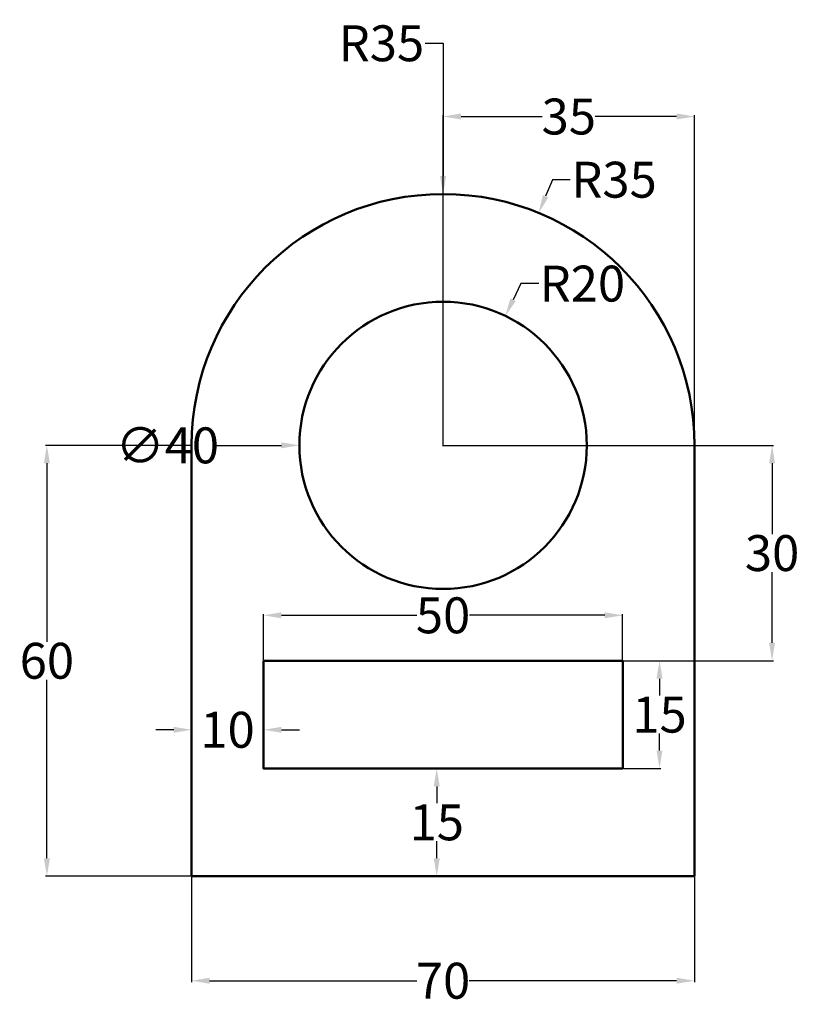
# Model space of a CAD drawing. Units: millimetres. Extents: x -34 to 74, y -57 to 80.
import ezdxf

# ---------------------------------------------------------------- set-up
doc = ezdxf.new("R2010")
doc.units = ezdxf.units.MM
doc.header["$MEASUREMENT"] = 0
doc.layers.add('M-DIMS', color=2, linetype='Continuous', lineweight=25)
doc.layers.add('M-OUTL', color=7, linetype='Continuous', lineweight=50)
doc.styles.get("Standard").update_dxf_attribs({"font": 'arial.ttf'})
doc.dimstyles.get("Standard").update_dxf_attribs({"dimtxt": 5, "dimasz": 2.5, "dimexe": 0.18, "dimexo": 0.1, "dimgap": 0.09, "dimtad": 0, "dimtih": 1, "dimtoh": 1, "dimdec": 4, "dimdsep": 46, "dimtxsty": 'Standard', "dimcen": 0.09, "dimclrd": 2, "dimclre": 2, "dimclrt": 2, "dimadec": 0, "dimazin": 0, "dimtfac": 1, "dimtdec": 4, "dimtofl": 0, "dimtmove": 0, "dimatfit": 3, "dimfxl": 1, "dimtfillclr": 2, "dimtolj": 1, "dimtzin": 0, "dimarcsym": 0})

# ---------------------------------------------------------------- blocks, each defined once
blk = doc.blocks.new('*D1')
at = {"layer": 'Defpoints', "color": 0, "transparency": 16777216}
for p in [(-10.41, -39.16), (59.59, -39.16), (59.59, -53.72)]:
    blk.add_point(p, dxfattribs=at)
at = {"layer": 'M-DIMS', "color": 0, "lineweight": -2, "transparency": 16777216}
for p, q in [((-10.41, -39.26), (-10.41, -53.9)), ((59.59, -39.26), (59.59, -53.9)), ((-7.91, -53.72), (20.95, -53.72)), ((57.09, -53.72), (28.23, -53.72))]:
    blk.add_line(p, q, dxfattribs=at)
at = {"layer": 'M-DIMS', "color": 0, "transparency": 16777216}
for points in [[(-7.91, -53.31), (-7.91, -54.14), (-10.41, -53.72)], [(57.09, -53.31), (57.09, -54.14), (59.59, -53.72)]]:
    blk.add_solid(points, dxfattribs=at)
at = {"layer": 'M-DIMS', "color": 0, "transparency": 16777216, "insert": (24.59, -53.72), "char_height": 5, "attachment_point": 5}
blk.add_mtext('\\A1;70', dxfattribs=at)
blk = doc.blocks.new('*D2')
at = {"layer": 'Defpoints', "color": 0, "transparency": 16777216}
for p in [(-30.56, 20.84), (-10.41, 20.84), (-10.41, -39.16)]:
    blk.add_point(p, dxfattribs=at)
at = {"layer": 'M-DIMS', "color": 0, "lineweight": -2, "transparency": 16777216}
for p, q in [((-10.51, 20.84), (-30.74, 20.84)), ((-30.56, 18.34), (-30.56, -6.51)), ((-30.56, -36.66), (-30.56, -11.8)), ((-10.51, -39.16), (-30.74, -39.16))]:
    blk.add_line(p, q, dxfattribs=at)
at = {"layer": 'M-DIMS', "color": 0, "transparency": 16777216}
for points in [[(-30.97, 18.34), (-30.14, 18.34), (-30.56, 20.84)], [(-30.97, -36.66), (-30.14, -36.66), (-30.56, -39.16)]]:
    blk.add_solid(points, dxfattribs=at)
at = {"layer": 'M-DIMS', "color": 0, "transparency": 16777216, "insert": (-30.56, -9.16), "char_height": 5, "attachment_point": 5}
blk.add_mtext('\\A1;60', dxfattribs=at)
blk = doc.blocks.new('*D3')
at = {"layer": 'Defpoints', "color": 0, "transparency": 16777216}
for p in [(49.59, -2.83), (-0.41, -9.16), (49.59, -9.16)]:
    blk.add_point(p, dxfattribs=at)
at = {"layer": 'M-DIMS', "color": 0, "lineweight": -2, "transparency": 16777216}
for p, q in [((-0.41, -9.06), (-0.41, -2.65)), ((49.59, -9.06), (49.59, -2.65)), ((2.09, -2.83), (20.93, -2.83)), ((47.09, -2.83), (28.25, -2.83))]:
    blk.add_line(p, q, dxfattribs=at)
at = {"layer": 'M-DIMS', "color": 0, "transparency": 16777216}
for points in [[(2.09, -2.41), (2.09, -3.24), (-0.41, -2.83)], [(47.09, -2.41), (47.09, -3.24), (49.59, -2.83)]]:
    blk.add_solid(points, dxfattribs=at)
at = {"layer": 'M-DIMS', "color": 0, "transparency": 16777216, "insert": (24.59, -2.83), "char_height": 5, "attachment_point": 5}
blk.add_mtext('\\A1;50', dxfattribs=at)
blk = doc.blocks.new('*D4')
at = {"layer": 'Defpoints', "color": 0, "transparency": 16777216}
for p in [(-10.41, -16.66), (-0.41, -16.66), (-10.41, -18.77)]:
    blk.add_point(p, dxfattribs=at)
at = {"layer": 'M-DIMS', "color": 0, "lineweight": -2, "transparency": 16777216}
for p, q in [((-10.41, -16.76), (-10.41, -18.95)), ((-0.41, -16.76), (-0.41, -18.95)), ((-12.91, -18.77), (-15.41, -18.77)), ((2.09, -18.77), (4.59, -18.77))]:
    blk.add_line(p, q, dxfattribs=at)
at = {"layer": 'M-DIMS', "color": 0, "transparency": 16777216}
for points in [[(-12.91, -18.36), (-12.91, -19.19), (-10.41, -18.77)], [(2.09, -18.36), (2.09, -19.19), (-0.41, -18.77)]]:
    blk.add_solid(points, dxfattribs=at)
at = {"layer": 'M-DIMS', "color": 0, "transparency": 16777216, "insert": (-5.41, -18.77), "char_height": 5, "attachment_point": 5}
blk.add_mtext('\\A1;10', dxfattribs=at)
blk = doc.blocks.new('*D5')
at = {"layer": 'Defpoints', "color": 0, "transparency": 16777216}
for p in [(24.59, -24.16), (23.71, -39.16), (24.59, -39.16)]:
    blk.add_point(p, dxfattribs=at)
at = {"layer": 'M-DIMS', "color": 0, "lineweight": -2, "transparency": 16777216}
for p, q in [((24.49, -24.16), (23.53, -24.16)), ((23.71, -26.66), (23.71, -29.01)), ((23.71, -36.66), (23.71, -34.3)), ((24.49, -39.16), (23.53, -39.16))]:
    blk.add_line(p, q, dxfattribs=at)
at = {"layer": 'M-DIMS', "color": 0, "transparency": 16777216}
for points in [[(23.29, -26.66), (24.13, -26.66), (23.71, -24.16)], [(23.29, -36.66), (24.13, -36.66), (23.71, -39.16)]]:
    blk.add_solid(points, dxfattribs=at)
at = {"layer": 'M-DIMS', "color": 0, "transparency": 16777216, "insert": (23.71, -31.66), "char_height": 5, "attachment_point": 5}
blk.add_mtext('\\A1;15', dxfattribs=at)
blk = doc.blocks.new('*D6')
at = {"layer": 'Defpoints', "color": 0, "transparency": 16777216}
for p in [(49.59, -9.16), (49.59, -24.16), (54.72, -24.16)]:
    blk.add_point(p, dxfattribs=at)
at = {"layer": 'M-DIMS', "color": 0, "lineweight": -2, "transparency": 16777216}
for p, q in [((49.69, -9.16), (54.9, -9.16)), ((54.72, -11.66), (54.72, -14.01)), ((54.72, -21.66), (54.72, -19.3)), ((49.69, -24.16), (54.9, -24.16))]:
    blk.add_line(p, q, dxfattribs=at)
at = {"layer": 'M-DIMS', "color": 0, "transparency": 16777216}
for points in [[(54.3, -11.66), (55.13, -11.66), (54.72, -9.16)], [(54.3, -21.66), (55.13, -21.66), (54.72, -24.16)]]:
    blk.add_solid(points, dxfattribs=at)
at = {"layer": 'M-DIMS', "color": 0, "transparency": 16777216, "insert": (54.72, -16.66), "char_height": 5, "attachment_point": 5}
blk.add_mtext('\\A1;15', dxfattribs=at)
blk = doc.blocks.new('*D7')
at = {"layer": 'Defpoints', "color": 0, "transparency": 16777216}
for p in [(33.26, 38.87), (24.59, 20.84)]:
    blk.add_point(p, dxfattribs=at)
at = {"layer": 'M-DIMS', "color": 0, "lineweight": -2, "transparency": 16777216}
for p, q in [((35.42, 43.37), (34.34, 41.12)), ((37.92, 43.37), (35.42, 43.37)), ((24.5, 20.84), (24.68, 20.84)), ((24.59, 20.75), (24.59, 20.93))]:
    blk.add_line(p, q, dxfattribs=at)
at = {"layer": 'M-DIMS', "color": 0, "transparency": 16777216}
blk.add_solid([(33.96, 41.3), (34.72, 40.94), (33.26, 38.87)], dxfattribs=at)
at = {"layer": 'M-DIMS', "color": 0, "transparency": 16777216, "insert": (43.98, 43.37), "char_height": 5, "attachment_point": 5}
blk.add_mtext('\\A1;R20', dxfattribs=at)
blk = doc.blocks.new('*D8')
at = {"layer": 'Defpoints', "color": 0, "transparency": 16777216}
for p in [(37.9, 53.21), (24.59, 20.84)]:
    blk.add_point(p, dxfattribs=at)
at = {"layer": 'M-DIMS', "color": 0, "lineweight": -2, "transparency": 16777216}
for p, q in [((39.8, 57.84), (38.85, 55.53)), ((42.3, 57.84), (39.8, 57.84)), ((24.5, 20.84), (24.68, 20.84)), ((24.59, 20.75), (24.59, 20.93))]:
    blk.add_line(p, q, dxfattribs=at)
at = {"layer": 'M-DIMS', "color": 0, "transparency": 16777216}
blk.add_solid([(38.47, 55.68), (39.24, 55.37), (37.9, 53.21)], dxfattribs=at)
at = {"layer": 'M-DIMS', "color": 0, "transparency": 16777216, "insert": (48.39, 57.84), "char_height": 5, "attachment_point": 5}
blk.add_mtext('\\A1;R35', dxfattribs=at)
blk = doc.blocks.new('*D9')
at = {"layer": 'Defpoints', "color": 0, "transparency": 16777216}
for p in [(59.59, 66.64), (24.59, 20.84), (59.59, 20.84)]:
    blk.add_point(p, dxfattribs=at)
at = {"layer": 'M-DIMS', "color": 2, "lineweight": -2, "transparency": 16777216}
for p, q in [((24.59, 20.94), (24.59, 66.82)), ((27.09, 66.64), (38.4, 66.64)), ((57.09, 66.64), (45.78, 66.64)), ((59.59, 20.94), (59.59, 66.82))]:
    blk.add_line(p, q, dxfattribs=at)
at = {"layer": 'M-DIMS', "color": 2, "transparency": 16777216}
for points in [[(27.09, 67.06), (27.09, 66.23), (24.59, 66.64)], [(57.09, 67.06), (57.09, 66.23), (59.59, 66.64)]]:
    blk.add_solid(points, dxfattribs=at)
at = {"layer": 'M-DIMS', "color": 2, "transparency": 16777216, "insert": (42.09, 66.64), "char_height": 5, "attachment_point": 5}
blk.add_mtext('\\A1;35', dxfattribs=at)
blk = doc.blocks.new('*D10')
at = {"layer": 'Defpoints', "color": 0, "transparency": 16777216}
for p in [(24.59, 20.84), (70.39, 20.84), (49.59, -9.16)]:
    blk.add_point(p, dxfattribs=at)
at = {"layer": 'M-DIMS', "color": 2, "lineweight": -2, "transparency": 16777216}
for p, q in [((24.69, 20.84), (70.57, 20.84)), ((70.39, 18.34), (70.39, 8.49)), ((70.39, -6.66), (70.39, 3.2)), ((49.69, -9.16), (70.57, -9.16))]:
    blk.add_line(p, q, dxfattribs=at)
at = {"layer": 'M-DIMS', "color": 2, "transparency": 16777216}
for points in [[(69.97, 18.34), (70.81, 18.34), (70.39, 20.84)], [(69.97, -6.66), (70.81, -6.66), (70.39, -9.16)]]:
    blk.add_solid(points, dxfattribs=at)
at = {"layer": 'M-DIMS', "color": 2, "transparency": 16777216, "insert": (70.39, 5.84), "char_height": 5, "attachment_point": 5}
blk.add_mtext('\\A1;30', dxfattribs=at)
blk = doc.blocks.new('*D11')
at = {"layer": 'Defpoints', "color": 0, "transparency": 16777216}
for p in [(24.59, 55.84), (24.59, 20.84)]:
    blk.add_point(p, dxfattribs=at)
at = {"layer": 'M-DIMS', "color": 2, "lineweight": -2, "transparency": 16777216}
for p, q in [((22.09, 76.84), (24.59, 76.84)), ((24.59, 76.84), (24.59, 58.34)), ((24.5, 20.84), (24.68, 20.84)), ((24.59, 20.75), (24.59, 20.93))]:
    blk.add_line(p, q, dxfattribs=at)
at = {"layer": 'M-DIMS', "color": 2, "transparency": 16777216}
blk.add_solid([(25.01, 58.34), (24.17, 58.34), (24.59, 55.84)], dxfattribs=at)
at = {"layer": 'M-DIMS', "color": 2, "transparency": 16777216, "insert": (16.01, 76.84), "char_height": 5, "attachment_point": 5}
blk.add_mtext('\\A1;R35', dxfattribs=at)
blk = doc.blocks.new('*D12')
at = {"layer": 'Defpoints', "color": 0, "transparency": 16777216}
for p in [(4.59, 20.84), (44.59, 20.84)]:
    blk.add_point(p, dxfattribs=at)
at = {"layer": 'M-DIMS', "color": 2, "lineweight": -2, "transparency": 16777216}
for p, q in [((-7.41, 20.84), (2.09, 20.84)), ((24.5, 20.84), (24.68, 20.84)), ((24.59, 20.75), (24.59, 20.93))]:
    blk.add_line(p, q, dxfattribs=at)
at = {"layer": 'M-DIMS', "color": 2, "transparency": 16777216}
blk.add_solid([(2.09, 21.26), (2.09, 20.43), (4.59, 20.84)], dxfattribs=at)
at = {"layer": 'M-DIMS', "color": 2, "transparency": 16777216, "insert": (-13.79, 20.84), "char_height": 5, "attachment_point": 5}
blk.add_mtext('\\A1;∅40', dxfattribs=at)

msp = doc.modelspace()

# ---------------------------------------------------------------- linework, layer by layer
at = {"layer": 'M-OUTL'}
for p, q in [((-10.40861, 20.84291), (-10.40861, -39.15709)), ((59.59139, -39.15709), (59.59139, 20.84291)), ((-10.40861, -39.15709), (59.59139, -39.15709))]:
    msp.add_line(p, q, dxfattribs=at)
msp.add_lwpolyline([(-0.40861, -9.15709), (49.59139, -9.15709), (49.59139, -24.15709), (-0.40861, -24.15709)], close=True, dxfattribs=at)
msp.add_circle((24.59139, 20.84291), 20, dxfattribs=at)
msp.add_arc((24.59139, 20.84291), 35, 0, 180, dxfattribs=at)

# ---------------------------------------------------------------- dimensions: what is measured, and where the dimension line sits
at = {"layer": 'M-DIMS'}
dim = msp.add_radius_dim(center=(24.59139, 20.84291), mpoint=(24.591, 55.84291), dimstyle='Standard', override={"dimdec": 0, "dimlfac": 1, "dimrnd": 0, "dimzin": 0, "dimdsep": 46, "dimlunit": 2}, dxfattribs=at)
dim.commit()
dim.dimension.update_dxf_attribs({"geometry": '*D11', "text_midpoint": (16.00827, 76.84291), "dimtype": 164})
for base, p1, p2, override, picture, middle in [((59.59139, 66.64291), (24.59139, 20.84291), (59.59139, 20.84291), {"dimdec": 0, "dimlfac": 1, "dimrnd": 0, "dimzin": 0, "dimdsep": 46, "dimlunit": 2}, '*D9', (42.09139, 66.64291)), ((49.59139, -2.82509), (-0.40861, -9.15709), (49.59139, -9.15709), {"dimclrd": 0, "dimclre": 0, "dimclrt": 0}, '*D3', (24.59139, -2.82509)), ((-10.40861, -18.77292), (-0.40861, -16.65709), (-10.40861, -16.65709), {"dimclrd": 0, "dimclre": 0, "dimclrt": 0}, '*D4', (-5.40861, -18.77292)), ((59.59139, -53.72273), (-10.40861, -39.15709), (59.59139, -39.15709), {"dimclrd": 0, "dimclre": 0, "dimclrt": 0}, '*D1', (24.59139, -53.72273))]:
    dim = msp.add_linear_dim(base=base, p1=p1, p2=p2, dimstyle='Standard', override=override, dxfattribs=at)
    dim.commit()
    dim.dimension.update_dxf_attribs({"geometry": picture, "text_midpoint": middle})
for mpoint, picture, middle in [((37.9024, 53.21291), '*D8', (48.38647, 57.83719)), ((33.25688, 38.86815), '*D7', (43.97847, 43.37446))]:
    dim = msp.add_radius_dim(center=(24.59139, 20.84291), mpoint=mpoint, dimstyle='Standard', override={"dimclrd": 0, "dimclre": 0, "dimclrt": 0}, dxfattribs=at)
    dim.commit()
    dim.dimension.update_dxf_attribs({"geometry": picture, "text_midpoint": middle})
dim = msp.add_diameter_dim_2p(p1=(44.59139, 20.84282), p2=(4.59139, 20.843), dimstyle='Standard', override={"dimdec": 0, "dimlfac": 1, "dimrnd": 0, "dimzin": 0, "dimdsep": 46, "dimlunit": 2}, dxfattribs=at)
dim.commit()
dim.dimension.update_dxf_attribs({"geometry": '*D12', "text_midpoint": (-7.40861, 20.84306), "dimtype": 163})
for base, p1, p2, override, picture, middle in [((-30.55717, 20.84291), (-10.40861, -39.15709), (-10.40861, 20.84291), {"dimclrd": 0, "dimclre": 0, "dimclrt": 0}, '*D2', (-30.55717, -9.15709)), ((70.39139, 20.84291), (49.59139, -9.15709), (24.59139, 20.84291), {"dimdec": 0, "dimlfac": 1, "dimrnd": 0, "dimzin": 0, "dimdsep": 46, "dimlunit": 2}, '*D10', (70.39139, 5.84291)), ((54.7181, -24.15709), (49.59139, -9.15709), (49.59139, -24.15709), {"dimclrd": 0, "dimclre": 0, "dimclrt": 0}, '*D6', (54.7181, -16.65709)), ((23.70891, -39.15709), (24.59139, -24.15709), (24.59139, -39.15709), {"dimclrd": 0, "dimclre": 0, "dimclrt": 0}, '*D5', (23.70891, -31.65709))]:
    dim = msp.add_linear_dim(base=base, p1=p1, p2=p2, angle=90, dimstyle='Standard', override=override, dxfattribs=at)
    dim.commit()
    dim.dimension.update_dxf_attribs({"geometry": picture, "text_midpoint": middle})

doc.saveas('drawing.dxf')
